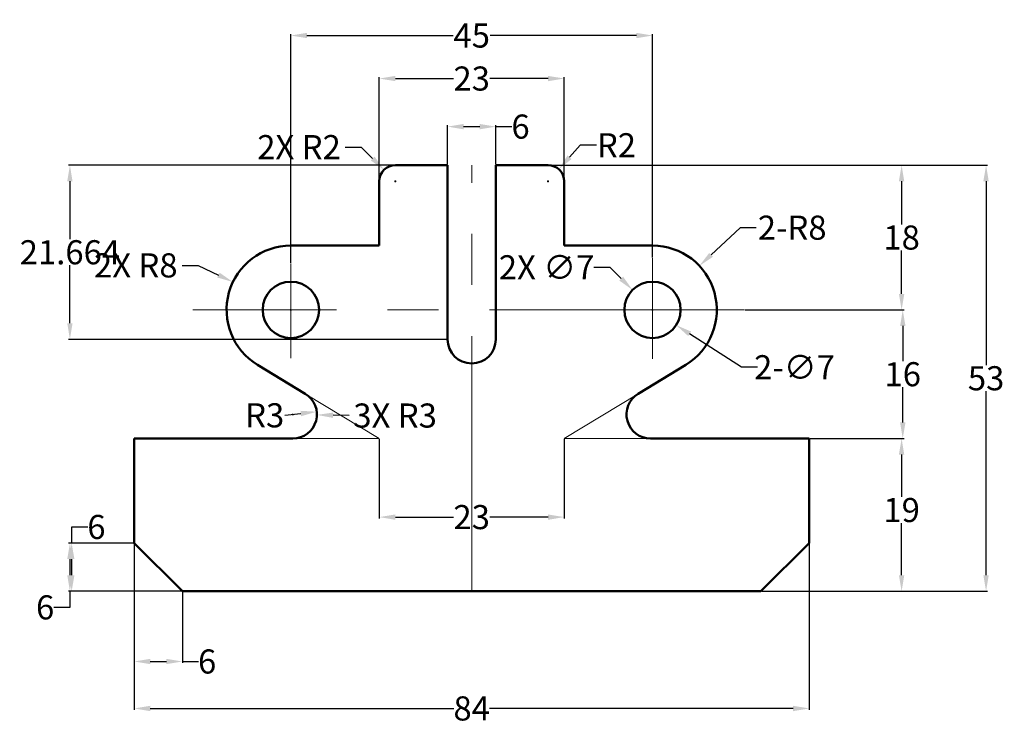
# Model space of a CAD drawing. Units: inches. Extents: x 46 to 168, y 15 to 102.
import ezdxf

# ---------------------------------------------------------------- set-up
doc = ezdxf.new("R2010")
doc.units = ezdxf.units.IN
doc.header["$MEASUREMENT"] = 0
doc.linetypes.add('ACAD_ISO04W100', pattern=[30, 24, -3, 0, -3])
doc.linetypes.add('CENTER', pattern=[50.8, 31.75, -6.35, 6.35, -6.35])
for name, color, linetype, lineweight in [('M-CNTR', 4, 'CENTER', 18), ('M-CONS', 4, 'ACAD_ISO04W100', 18), ('M-DIMS', 2, 'Continuous', 25), ('M-OUTL', 7, 'Continuous', 50)]:
    doc.layers.add(name, color=color, linetype=linetype, lineweight=lineweight)
doc.styles.get("Standard").update_dxf_attribs({"font": 'arial.ttf'})
doc.dimstyles.get("Standard").update_dxf_attribs({"dimtxt": 3, "dimasz": 2, "dimexe": 0.18, "dimexo": 0.0625, "dimgap": 0.09, "dimtad": 0, "dimtih": 1, "dimtoh": 1, "dimdec": 0, "dimzin": 0, "dimdsep": 46, "dimtxsty": 'Standard', "dimcen": 0.09, "dimclrd": 1, "dimclre": 1, "dimadec": 0, "dimazin": 0, "dimtfac": 1, "dimtdec": 0, "dimtofl": 0, "dimtmove": 0, "dimatfit": 3, "dimfxl": 1, "dimtolj": 1, "dimtzin": 0, "dimarcsym": 0})

# ---------------------------------------------------------------- blocks, each defined once
blk = doc.blocks.new('*D1')
at = {"layer": 'Defpoints', "color": 0, "transparency": 16777216}
for p in [(144.16, 50.26), (138.16, 31.26), (155.66, 31.26)]:
    blk.add_point(p, dxfattribs=at)
at = {"layer": 'M-DIMS', "color": 0, "lineweight": -2, "transparency": 16777216}
for p, q in [((144.22, 50.26), (155.84, 50.26)), ((155.66, 48.26), (155.66, 42.99)), ((155.66, 33.26), (155.66, 39.75)), ((138.22, 31.26), (155.84, 31.26))]:
    blk.add_line(p, q, dxfattribs=at)
at = {"layer": 'M-DIMS', "color": 0, "transparency": 16777216}
for points in [[(155.32, 48.26), (155.99, 48.26), (155.66, 50.26)], [(155.32, 33.26), (155.99, 33.26), (155.66, 31.26)]]:
    blk.add_solid(points, dxfattribs=at)
at = {"layer": 'M-DIMS', "color": 0, "transparency": 16777216, "insert": (155.66, 41.37), "char_height": 3, "attachment_point": 5}
blk.add_mtext('\\A1;19', dxfattribs=at)
blk = doc.blocks.new('*D2')
at = {"layer": 'Defpoints', "color": 0, "transparency": 16777216}
for p in [(60.16, 37.26), (66.16, 31.26), (66.16, 22.53)]:
    blk.add_point(p, dxfattribs=at)
at = {"layer": 'M-DIMS', "color": 0, "lineweight": -2, "transparency": 16777216}
for p, q in [((60.16, 37.2), (60.16, 22.35)), ((66.16, 31.2), (66.16, 22.35)), ((62.16, 22.53), (64.16, 22.53)), ((66.16, 22.53), (68.16, 22.53))]:
    blk.add_line(p, q, dxfattribs=at)
at = {"layer": 'M-DIMS', "color": 0, "transparency": 16777216}
for points in [[(62.16, 22.86), (62.16, 22.2), (60.16, 22.53)], [(64.16, 22.86), (64.16, 22.2), (66.16, 22.53)]]:
    blk.add_solid(points, dxfattribs=at)
at = {"layer": 'M-DIMS', "color": 0, "transparency": 16777216, "insert": (69.24, 22.53), "char_height": 3, "attachment_point": 5}
blk.add_mtext('\\A1;6', dxfattribs=at)
blk = doc.blocks.new('*D3')
at = {"layer": 'Defpoints', "color": 0, "transparency": 16777216}
for p in [(52.38, 37.26), (60.16, 37.26), (66.16, 31.26)]:
    blk.add_point(p, dxfattribs=at)
at = {"layer": 'M-DIMS', "color": 0, "lineweight": -2, "transparency": 16777216}
for p, q in [((52.38, 37.26), (52.38, 39.26)), ((52.38, 39.26), (54.38, 39.26)), ((60.1, 37.26), (52.2, 37.26)), ((52.38, 33.26), (52.38, 35.26)), ((66.1, 31.26), (52.2, 31.26))]:
    blk.add_line(p, q, dxfattribs=at)
at = {"layer": 'M-DIMS', "color": 0, "transparency": 16777216}
for points in [[(52.05, 35.26), (52.72, 35.26), (52.38, 37.26)], [(52.05, 33.26), (52.72, 33.26), (52.38, 31.26)]]:
    blk.add_solid(points, dxfattribs=at)
at = {"layer": 'M-DIMS', "color": 0, "transparency": 16777216, "insert": (55.46, 39.26), "char_height": 3, "attachment_point": 5}
blk.add_mtext('\\A1;6', dxfattribs=at)
blk = doc.blocks.new('*D4')
at = {"layer": 'Defpoints', "color": 0, "transparency": 16777216}
for p in [(136.12, 66.26), (144.16, 50.26), (155.8, 50.26)]:
    blk.add_point(p, dxfattribs=at)
at = {"layer": 'M-DIMS', "color": 0, "lineweight": -2, "transparency": 16777216}
for p, q in [((136.18, 66.26), (155.98, 66.26)), ((155.8, 64.26), (155.8, 59.89)), ((155.8, 52.26), (155.8, 56.64)), ((144.22, 50.26), (155.98, 50.26))]:
    blk.add_line(p, q, dxfattribs=at)
at = {"layer": 'M-DIMS', "color": 0, "transparency": 16777216}
for points in [[(155.47, 64.26), (156.14, 64.26), (155.8, 66.26)], [(155.47, 52.26), (156.14, 52.26), (155.8, 50.26)]]:
    blk.add_solid(points, dxfattribs=at)
at = {"layer": 'M-DIMS', "color": 0, "transparency": 16777216, "insert": (155.8, 58.26), "char_height": 3, "attachment_point": 5}
blk.add_mtext('\\A1;16', dxfattribs=at)
blk = doc.blocks.new('*D5')
at = {"layer": 'Defpoints', "color": 0, "transparency": 16777216}
for p in [(111.66, 84.26), (136.12, 66.26), (155.66, 66.26)]:
    blk.add_point(p, dxfattribs=at)
at = {"layer": 'M-DIMS', "color": 0, "lineweight": -2, "transparency": 16777216}
for p, q in [((111.72, 84.26), (155.84, 84.26)), ((155.66, 82.26), (155.66, 76.89)), ((155.66, 68.26), (155.66, 73.64)), ((136.18, 66.26), (155.84, 66.26))]:
    blk.add_line(p, q, dxfattribs=at)
at = {"layer": 'M-DIMS', "color": 0, "transparency": 16777216}
for points in [[(155.32, 82.26), (155.99, 82.26), (155.66, 84.26)], [(155.32, 68.26), (155.99, 68.26), (155.66, 66.26)]]:
    blk.add_solid(points, dxfattribs=at)
at = {"layer": 'M-DIMS', "color": 0, "transparency": 16777216, "insert": (155.66, 75.26), "char_height": 3, "attachment_point": 5}
blk.add_mtext('\\A1;18', dxfattribs=at)
blk = doc.blocks.new('*D6')
at = {"layer": 'Defpoints', "color": 0, "transparency": 16777216}
for p in [(105.16, 89.06), (99.16, 84.26), (105.16, 84.26)]:
    blk.add_point(p, dxfattribs=at)
at = {"layer": 'M-DIMS', "color": 0, "lineweight": -2, "transparency": 16777216}
for p, q in [((99.16, 84.33), (99.16, 89.24)), ((101.16, 89.06), (103.16, 89.06)), ((105.16, 84.33), (105.16, 89.24)), ((105.16, 89.06), (107.16, 89.06))]:
    blk.add_line(p, q, dxfattribs=at)
at = {"layer": 'M-DIMS', "color": 0, "transparency": 16777216}
for points in [[(101.16, 89.39), (101.16, 88.72), (99.16, 89.06)], [(103.16, 89.39), (103.16, 88.72), (105.16, 89.06)]]:
    blk.add_solid(points, dxfattribs=at)
at = {"layer": 'M-DIMS', "color": 0, "transparency": 16777216, "insert": (108.24, 89.06), "char_height": 3, "attachment_point": 5}
blk.add_mtext('\\A1;6', dxfattribs=at)
blk = doc.blocks.new('*D7')
at = {"layer": 'Defpoints', "color": 0, "transparency": 16777216}
for p in [(111.66, 84.26), (138.16, 31.26), (166.17, 31.26)]:
    blk.add_point(p, dxfattribs=at)
at = {"layer": 'M-DIMS', "color": 0, "lineweight": -2, "transparency": 16777216}
for p, q in [((111.72, 84.26), (166.35, 84.26)), ((166.17, 82.26), (166.17, 59.39)), ((166.17, 33.26), (166.17, 56.14)), ((138.22, 31.26), (166.35, 31.26))]:
    blk.add_line(p, q, dxfattribs=at)
at = {"layer": 'M-DIMS', "color": 0, "transparency": 16777216}
for points in [[(165.83, 82.26), (166.5, 82.26), (166.17, 84.26)], [(165.83, 33.26), (166.5, 33.26), (166.17, 31.26)]]:
    blk.add_solid(points, dxfattribs=at)
at = {"layer": 'M-DIMS', "color": 0, "transparency": 16777216, "insert": (166.17, 57.76), "char_height": 3, "attachment_point": 5}
blk.add_mtext('\\A1;53', dxfattribs=at)
blk = doc.blocks.new('*D8')
at = {"layer": 'Defpoints', "color": 0, "transparency": 16777216}
for p in [(130.49, 71.74), (124.66, 66.26)]:
    blk.add_point(p, dxfattribs=at)
at = {"layer": 'M-DIMS', "color": 0, "lineweight": -2, "transparency": 16777216}
for p, q in [((135.56, 76.49), (131.95, 73.1)), ((137.56, 76.49), (135.56, 76.49)), ((124.57, 66.26), (124.75, 66.26)), ((124.66, 66.17), (124.66, 66.35))]:
    blk.add_line(p, q, dxfattribs=at)
at = {"layer": 'M-DIMS', "color": 0, "transparency": 16777216}
blk.add_solid([(131.72, 73.35), (132.18, 72.86), (130.49, 71.74)], dxfattribs=at)
at = {"layer": 'M-DIMS', "color": 0, "transparency": 16777216, "insert": (142.04, 76.49), "char_height": 3, "attachment_point": 5}
blk.add_mtext('\\A1;2-R8', dxfattribs=at)
blk = doc.blocks.new('*D9')
at = {"layer": 'Defpoints', "color": 0, "transparency": 16777216}
for p in [(121.72, 68.16), (127.6, 64.37)]:
    blk.add_point(p, dxfattribs=at)
at = {"layer": 'M-DIMS', "color": 0, "lineweight": -2, "transparency": 16777216}
for p, q in [((124.57, 66.26), (124.75, 66.26)), ((124.66, 66.17), (124.66, 66.35)), ((135.73, 59.13), (129.28, 63.29)), ((137.73, 59.13), (135.73, 59.13))]:
    blk.add_line(p, q, dxfattribs=at)
at = {"layer": 'M-DIMS', "color": 0, "transparency": 16777216}
blk.add_solid([(129.46, 63.57), (129.1, 63.01), (127.6, 64.37)], dxfattribs=at)
at = {"layer": 'M-DIMS', "color": 0, "transparency": 16777216, "insert": (142.33, 59.13), "char_height": 3, "attachment_point": 5}
blk.add_mtext('\\A1;2-∅7', dxfattribs=at)
blk = doc.blocks.new('*D10')
at = {"layer": 'Defpoints', "color": 0, "transparency": 16777216}
for p in [(60.16, 37.26), (144.16, 37.26), (144.16, 16.69)]:
    blk.add_point(p, dxfattribs=at)
at = {"layer": 'M-DIMS', "color": 0, "lineweight": -2, "transparency": 16777216}
for p, q in [((60.16, 37.2), (60.16, 16.51)), ((144.16, 37.2), (144.16, 16.51)), ((62.16, 16.69), (99.92, 16.69)), ((142.16, 16.69), (104.39, 16.69))]:
    blk.add_line(p, q, dxfattribs=at)
at = {"layer": 'M-DIMS', "color": 0, "transparency": 16777216}
for points in [[(62.16, 17.02), (62.16, 16.35), (60.16, 16.69)], [(142.16, 17.02), (142.16, 16.35), (144.16, 16.69)]]:
    blk.add_solid(points, dxfattribs=at)
at = {"layer": 'M-DIMS', "color": 0, "transparency": 16777216, "insert": (102.16, 16.69), "char_height": 3, "attachment_point": 5}
blk.add_mtext('\\A1;84', dxfattribs=at)
blk = doc.blocks.new('*D11')
at = {"layer": 'Defpoints', "color": 0, "transparency": 16777216}
for p in [(124.66, 100.39), (124.66, 72.7), (79.66, 72.05)]:
    blk.add_point(p, dxfattribs=at)
at = {"layer": 'M-DIMS', "color": 0, "lineweight": -2, "transparency": 16777216}
for p, q in [((79.66, 72.12), (79.66, 100.57)), ((124.66, 72.76), (124.66, 100.57)), ((81.66, 100.39), (99.85, 100.39)), ((122.66, 100.39), (104.47, 100.39))]:
    blk.add_line(p, q, dxfattribs=at)
at = {"layer": 'M-DIMS', "color": 0, "transparency": 16777216}
for points in [[(81.66, 100.72), (81.66, 100.06), (79.66, 100.39)], [(122.66, 100.72), (122.66, 100.06), (124.66, 100.39)]]:
    blk.add_solid(points, dxfattribs=at)
at = {"layer": 'M-DIMS', "color": 0, "transparency": 16777216, "insert": (102.16, 100.39), "char_height": 3, "attachment_point": 5}
blk.add_mtext('\\A1;45', dxfattribs=at)
blk = doc.blocks.new('*D12')
at = {"layer": 'Defpoints', "color": 0, "transparency": 16777216}
for p in [(113.66, 95.04), (90.66, 82.26), (113.66, 82.26)]:
    blk.add_point(p, dxfattribs=at)
at = {"layer": 'M-DIMS', "color": 0, "lineweight": -2, "transparency": 16777216}
for p, q in [((90.66, 82.33), (90.66, 95.22)), ((92.66, 95.04), (99.89, 95.04)), ((111.66, 95.04), (104.42, 95.04)), ((113.66, 82.33), (113.66, 95.22))]:
    blk.add_line(p, q, dxfattribs=at)
at = {"layer": 'M-DIMS', "color": 0, "transparency": 16777216}
for points in [[(92.66, 95.37), (92.66, 94.71), (90.66, 95.04)], [(111.66, 95.37), (111.66, 94.71), (113.66, 95.04)]]:
    blk.add_solid(points, dxfattribs=at)
at = {"layer": 'M-DIMS', "color": 0, "transparency": 16777216, "insert": (102.16, 95.04), "char_height": 3, "attachment_point": 5}
blk.add_mtext('\\A1;23', dxfattribs=at)
blk = doc.blocks.new('*D13')
at = {"layer": 'Defpoints', "color": 0, "transparency": 16777216}
for p in [(112.99, 83.75), (111.66, 82.26)]:
    blk.add_point(p, dxfattribs=at)
at = {"layer": 'M-DIMS', "color": 0, "lineweight": -2, "transparency": 16777216}
for p, q in [((115.67, 86.74), (114.33, 85.24)), ((117.67, 86.74), (115.67, 86.74)), ((111.57, 82.26), (111.75, 82.26)), ((111.66, 82.17), (111.66, 82.35))]:
    blk.add_line(p, q, dxfattribs=at)
at = {"layer": 'M-DIMS', "color": 0, "transparency": 16777216}
blk.add_solid([(114.08, 85.47), (114.58, 85.02), (112.99, 83.75)], dxfattribs=at)
at = {"layer": 'M-DIMS', "color": 0, "transparency": 16777216, "insert": (120.17, 86.74), "char_height": 3, "attachment_point": 5}
blk.add_mtext('\\A1;R2', dxfattribs=at)
blk = doc.blocks.new('*D14')
at = {"layer": 'Defpoints', "color": 0, "transparency": 16777216}
for p in [(90.66, 50.26), (113.66, 50.26), (113.66, 40.49)]:
    blk.add_point(p, dxfattribs=at)
at = {"layer": 'M-DIMS', "color": 0, "lineweight": -2, "transparency": 16777216}
for p, q in [((90.66, 50.2), (90.66, 40.31)), ((113.66, 50.2), (113.66, 40.31)), ((92.66, 40.49), (99.89, 40.49)), ((111.66, 40.49), (104.42, 40.49))]:
    blk.add_line(p, q, dxfattribs=at)
at = {"layer": 'M-DIMS', "color": 0, "transparency": 16777216}
for points in [[(92.66, 40.82), (92.66, 40.15), (90.66, 40.49)], [(111.66, 40.82), (111.66, 40.15), (113.66, 40.49)]]:
    blk.add_solid(points, dxfattribs=at)
at = {"layer": 'M-DIMS', "color": 0, "transparency": 16777216, "insert": (102.16, 40.49), "char_height": 3, "attachment_point": 5}
blk.add_mtext('\\A1;23', dxfattribs=at)
blk = doc.blocks.new('*D15')
at = {"layer": 'Defpoints', "color": 0, "transparency": 16777216}
for p in [(79.9, 53.26), (82.88, 53.6)]:
    blk.add_point(p, dxfattribs=at)
at = {"layer": 'M-DIMS', "color": 0, "lineweight": -2, "transparency": 16777216}
blk.add_line((78.91, 53.15), (80.89, 53.37), dxfattribs=at)
at = {"layer": 'M-DIMS', "color": 0, "transparency": 16777216}
blk.add_solid([(80.86, 53.71), (80.93, 53.04), (82.88, 53.6)], dxfattribs=at)
at = {"layer": 'M-DIMS', "color": 0, "transparency": 16777216, "insert": (76.4, 53.15), "char_height": 3, "attachment_point": 5}
blk.add_mtext('\\A1;R3', dxfattribs=at)
blk = doc.blocks.new('LINK-THRU-HOLE-D7')
blk.add_circle((3.5, 3.5), 3.5)
blk = doc.blocks.new('*D17')
at = {"layer": 'Defpoints', "color": 0, "transparency": 16777216}
for p in [(99.16, 84.26), (52.16, 62.6), (99.16, 62.6)]:
    blk.add_point(p, dxfattribs=at)
at = {"layer": 'M-DIMS', "color": 1, "lineweight": -2, "transparency": 16777216}
for p, q in [((99.1, 84.26), (51.98, 84.26)), ((52.16, 82.26), (52.16, 75.05)), ((52.16, 64.6), (52.16, 71.81)), ((99.1, 62.6), (51.98, 62.6))]:
    blk.add_line(p, q, dxfattribs=at)
at = {"layer": 'M-DIMS', "color": 1, "transparency": 16777216}
for points in [[(51.83, 82.26), (52.49, 82.26), (52.16, 84.26)], [(51.83, 64.6), (52.49, 64.6), (52.16, 62.6)]]:
    blk.add_solid(points, dxfattribs=at)
at = {"layer": 'M-DIMS', "color": 0, "transparency": 16777216, "insert": (52.16, 73.43), "char_height": 3, "attachment_point": 5}
blk.add_mtext('\\A1;21.664', dxfattribs=at)
blk = doc.blocks.new('*D18')
at = {"layer": 'Defpoints', "color": 0, "transparency": 16777216}
for p in [(60.16, 37.26), (52.16, 31.26), (66.16, 31.26)]:
    blk.add_point(p, dxfattribs=at)
at = {"layer": 'M-DIMS', "color": 1, "lineweight": -2, "transparency": 16777216}
for p, q in [((60.1, 37.26), (51.98, 37.26)), ((52.16, 35.26), (52.16, 33.26)), ((66.1, 31.26), (51.98, 31.26)), ((52.16, 31.26), (52.16, 29.26)), ((52.16, 29.26), (50.16, 29.26))]:
    blk.add_line(p, q, dxfattribs=at)
at = {"layer": 'M-DIMS', "color": 1, "transparency": 16777216}
for points in [[(51.83, 35.26), (52.49, 35.26), (52.16, 37.26)], [(51.83, 33.26), (52.49, 33.26), (52.16, 31.26)]]:
    blk.add_solid(points, dxfattribs=at)
at = {"layer": 'M-DIMS', "color": 0, "transparency": 16777216, "insert": (49.08, 29.26), "char_height": 3, "attachment_point": 5}
blk.add_mtext('\\A1;6', dxfattribs=at)
blk = doc.blocks.new('*D19')
at = {"layer": 'Defpoints', "color": 0, "transparency": 16777216}
for p in [(72.45, 69.73), (79.66, 66.26)]:
    blk.add_point(p, dxfattribs=at)
at = {"layer": 'M-DIMS', "color": 1, "lineweight": -2, "transparency": 16777216}
for p, q in [((66.12, 71.8), (68.12, 71.8)), ((68.12, 71.8), (70.64, 70.59)), ((79.57, 66.26), (79.75, 66.26)), ((79.66, 66.17), (79.66, 66.35))]:
    blk.add_line(p, q, dxfattribs=at)
at = {"layer": 'M-DIMS', "color": 1, "transparency": 16777216}
blk.add_solid([(70.79, 70.89), (70.5, 70.29), (72.45, 69.73)], dxfattribs=at)
at = {"layer": 'M-DIMS', "color": 0, "transparency": 16777216, "insert": (60.36, 71.8), "char_height": 3, "attachment_point": 5}
blk.add_mtext('\\A1;2X R8', dxfattribs=at)
blk = doc.blocks.new('*D20')
at = {"layer": 'Defpoints', "color": 0, "transparency": 16777216}
for p in [(122.18, 68.74), (127.14, 63.79)]:
    blk.add_point(p, dxfattribs=at)
at = {"layer": 'M-DIMS', "color": 1, "lineweight": -2, "transparency": 16777216}
for p, q in [((117.35, 71.56), (119.35, 71.56)), ((119.35, 71.56), (120.77, 70.15)), ((124.57, 66.26), (124.75, 66.26)), ((124.66, 66.17), (124.66, 66.35))]:
    blk.add_line(p, q, dxfattribs=at)
at = {"layer": 'M-DIMS', "color": 1, "transparency": 16777216}
blk.add_solid([(121, 70.39), (120.53, 69.91), (122.18, 68.74)], dxfattribs=at)
at = {"layer": 'M-DIMS', "color": 0, "transparency": 16777216, "insert": (111.48, 71.56), "char_height": 3, "attachment_point": 5}
blk.add_mtext('\\A1;2X ∅7', dxfattribs=at)
blk = doc.blocks.new('*D21')
at = {"layer": 'Defpoints', "color": 0, "transparency": 16777216}
for p in [(79.9, 53.26), (82.9, 53.2)]:
    blk.add_point(p, dxfattribs=at)
at = {"layer": 'M-DIMS', "color": 1, "lineweight": -2, "transparency": 16777216}
for p, q in [((79.81, 53.26), (79.99, 53.26)), ((79.9, 53.17), (79.9, 53.35)), ((86.9, 53.12), (84.9, 53.16))]:
    blk.add_line(p, q, dxfattribs=at)
at = {"layer": 'M-DIMS', "color": 1, "transparency": 16777216}
blk.add_solid([(84.91, 53.49), (84.89, 52.83), (82.9, 53.2)], dxfattribs=at)
at = {"layer": 'M-DIMS', "color": 0, "transparency": 16777216, "insert": (92.63, 53.12), "char_height": 3, "attachment_point": 5}
blk.add_mtext('\\A1;3X R3', dxfattribs=at)
blk = doc.blocks.new('*D22')
at = {"layer": 'Defpoints', "color": 0, "transparency": 16777216}
for p in [(91.24, 83.68), (92.66, 82.26)]:
    blk.add_point(p, dxfattribs=at)
at = {"layer": 'M-DIMS', "color": 1, "lineweight": -2, "transparency": 16777216}
for p, q in [((86.42, 86.51), (88.42, 86.51)), ((88.42, 86.51), (89.83, 85.09)), ((92.57, 82.26), (92.75, 82.26)), ((92.66, 82.17), (92.66, 82.35))]:
    blk.add_line(p, q, dxfattribs=at)
at = {"layer": 'M-DIMS', "color": 1, "transparency": 16777216}
blk.add_solid([(90.07, 85.33), (89.59, 84.86), (91.24, 83.68)], dxfattribs=at)
at = {"layer": 'M-DIMS', "color": 0, "transparency": 16777216, "insert": (80.67, 86.51), "char_height": 3, "attachment_point": 5}
blk.add_mtext('\\A1;2X R2', dxfattribs=at)

msp = doc.modelspace()

# ---------------------------------------------------------------- linework, layer by layer
at = {"layer": 'M-CNTR'}
for p, q in [((102.1592, 31.2639), (102.1592, 84.2639)), ((124.6592, 60.1911), (124.6592, 72.6961)), ((79.6592, 60.2495), (79.6592, 72.0533)), ((136.1203, 66.2639), (67.441, 66.2639))]:
    msp.add_line(p, q, dxfattribs=at)
at = {"layer": 'M-CONS'}
for p, q in [((81.452, 55.8311), (90.6592, 50.2639)), ((122.8663, 55.8311), (113.6592, 50.2639)), ((79.8997, 50.2639), (90.6592, 50.2639)), ((124.4186, 50.2639), (113.6592, 50.2639))]:
    msp.add_line(p, q, dxfattribs=at)
at = {"layer": 'M-OUTL'}
for p, q in [((99.1592, 66.2639), (99.1592, 84.2639)), ((105.1592, 66.2639), (105.1592, 84.2639)), ((105.1592, 84.2639), (111.6592, 84.2639)), ((113.6592, 82.2639), (113.6592, 74.2639)), ((79.6592, 74.2639), (90.6592, 74.2639)), ((124.6592, 74.2639), (113.6592, 74.2639)), ((99.1592, 66.2639), (99.1592, 62.6004)), ((105.1592, 66.2639), (105.1592, 62.6004)), ((81.452, 55.8311), (75.5198, 59.4181)), ((122.8663, 55.8311), (128.7985, 59.4181)), ((60.1592, 37.2639), (60.1592, 50.2639)), ((60.1592, 50.2639), (79.8997, 50.2639)), ((144.1592, 50.2639), (124.4186, 50.2639)), ((144.1592, 37.2639), (144.1592, 50.2639)), ((66.1592, 31.2639), (60.1592, 37.2639)), ((138.1592, 31.2639), (144.1592, 37.2639)), ((66.1592, 31.2639), (138.1592, 31.2639))]:
    msp.add_line(p, q, dxfattribs=at)
msp.add_lwpolyline([(99.1592, 84.2639), (94.6592, 84.2639), (92.6592, 84.2639, 0.41421356), (90.6592, 82.2639), (90.6592, 80.2639), (90.6592, 74.2639)], format="xyb", dxfattribs=at)
for centre, radius, start, end in [((111.6592, 82.2639), 2, 0, 90), ((79.6592, 66.2639), 8, 90, 238.840375), ((124.6592, 66.2639), 8, 301.159625, 90), ((102.1592, 62.6004), 3, 180, 0), ((79.8997, 53.2639), 3, 270, 58.840375), ((124.4186, 53.2639), 3, 121.159625, 270)]:
    msp.add_arc(centre, radius, start, end, dxfattribs=at)

# ---------------------------------------------------------------- block references
for p in [(76.159, 62.764), (121.159, 62.764)]:
    msp.add_blockref('LINK-THRU-HOLE-D7', p, dxfattribs=at)

# ---------------------------------------------------------------- dimensions: what is measured, and where the dimension line sits
at = {"layer": 'M-DIMS'}
for base, p1, p2, picture, middle in [((124.6592, 100.3893), (79.6592, 72.0533), (124.6592, 72.6961), '*D11', (102.1592, 100.3893)), ((113.6592, 95.0417), (90.6592, 82.2639), (113.6592, 82.2639), '*D12', (102.1592, 95.0417)), ((113.6592, 40.4852), (90.6592, 50.2639), (113.6592, 50.2639), '*D14', (102.1592, 40.4852)), ((66.1592, 22.5292), (60.1592, 37.2639), (66.1592, 31.2639), '*D2', (69.2396, 22.5292)), ((144.1592, 16.6859), (60.1592, 37.2639), (144.1592, 37.2639), '*D10', (102.1592, 16.6859))]:
    dim = msp.add_linear_dim(base=base, p1=p1, p2=p2, dimstyle='Standard', override={"dimclrd": 0, "dimclre": 0, "dimclrt": 0}, dxfattribs=at)
    dim.commit()
    dim.dimension.update_dxf_attribs({"geometry": picture, "text_midpoint": middle})
for center, mpoint, text, picture, middle in [((92.6592, 82.2639), (91.2449, 83.6781), '2X <>', '*D22', (80.6743, 86.5064)), ((79.8997, 53.2639), (82.8991, 53.2021), '3X <>', '*D21', (92.6291, 53.1196))]:
    dim = msp.add_radius_dim(center=center, mpoint=mpoint, text=text, dimstyle='Standard', override={"dimdec": 0, "dimlfac": 1, "dimrnd": 0, "dimzin": 0, "dimdsep": 46, "dimlunit": 2}, dxfattribs=at)
    dim.commit()
    dim.dimension.update_dxf_attribs({"geometry": picture, "text_midpoint": middle})
for base, p1, p2, angle, override, picture, middle in [((105.1592, 89.0577), (99.1592, 84.2639), (105.1592, 84.2639), 180, {"dimclrd": 0, "dimclre": 0, "dimclrt": 0}, '*D6', (108.2396, 89.0577)), ((52.15915, 62.6004), (99.15915, 84.26393), (99.15915, 62.60039), 90, {"dimdec": 3, "dimlfac": 1, "dimrnd": 0, "dimzin": 0, "dimdsep": 46, "dimlunit": 2}, '*D17', (52.15915, 73.43216)), ((52.1592, 31.2639), (60.1592, 37.2639), (66.1592, 31.2639), 90, {"dimdec": 0, "dimlfac": 1, "dimrnd": 0, "dimzin": 0, "dimdsep": 46, "dimlunit": 2}, '*D18', (49.0787, 29.2639))]:
    dim = msp.add_linear_dim(base=base, p1=p1, p2=p2, angle=angle, dimstyle='Standard', override=override, dxfattribs=at)
    dim.commit()
    dim.dimension.update_dxf_attribs({"geometry": picture, "text_midpoint": middle})
for center, mpoint, picture, middle in [((111.6592, 82.2639), (112.994, 83.7533), '*D13', (120.1665, 86.7425)), ((79.8997, 53.2639), (82.8812, 53.5965), '*D15', (78.9059, 53.1531))]:
    dim = msp.add_radius_dim(center=center, mpoint=mpoint, dimstyle='Standard', override={"dimclrd": 0, "dimclre": 0, "dimclrt": 0}, dxfattribs=at)
    dim.commit()
    dim.dimension.update_dxf_attribs({"geometry": picture, "text_midpoint": middle, "dimtype": 164})
for base, p1, p2, picture, middle in [((155.6557, 66.2639), (111.6592, 84.2639), (136.1203, 66.2639), '*D5', (155.6557, 75.2639)), ((166.1663, 31.2639), (111.6592, 84.2639), (138.1592, 31.2639), '*D7', (166.1663, 57.7639)), ((155.8017, 50.2639), (136.1203, 66.2639), (144.1592, 50.2639), '*D4', (155.8017, 58.2639)), ((155.6557, 31.2639), (144.1592, 50.2639), (138.1592, 31.2639), '*D1', (155.6557, 41.3732)), ((52.3829, 37.2639), (66.1592, 31.2639), (60.1592, 37.2639), '*D3', (55.4633, 39.2639))]:
    dim = msp.add_linear_dim(base=base, p1=p1, p2=p2, angle=90, dimstyle='Standard', override={"dimclrd": 0, "dimclre": 0, "dimclrt": 0}, dxfattribs=at)
    dim.commit()
    dim.dimension.update_dxf_attribs({"geometry": picture, "text_midpoint": middle, "dimtype": 160})
for center, mpoint, text, override, picture, middle in [((124.6592, 66.2639), (130.4942, 71.7368), '2-<>', {"dimclrd": 0, "dimclre": 0, "dimclrt": 0}, '*D8', (142.0431, 76.4924)), ((79.6592, 66.2639), (72.4468, 69.7255), '2X <>', {"dimdec": 0, "dimlfac": 1, "dimrnd": 0, "dimzin": 0, "dimdsep": 46, "dimlunit": 2}, '*D19', (60.3589, 71.8025))]:
    dim = msp.add_radius_dim(center=center, mpoint=mpoint, text=text, dimstyle='Standard', override=override, dxfattribs=at)
    dim.commit()
    dim.dimension.update_dxf_attribs({"geometry": picture, "text_midpoint": middle, "dimtype": 164})
for p1, p2, text, override, picture, middle in [((127.1356, 63.7906), (122.1827, 68.7373), '2X <>', {"dimdec": 0, "dimlfac": 1, "dimrnd": 0, "dimzin": 0, "dimdsep": 46, "dimlunit": 2}, '*D20', (111.4784, 71.5639)), ((121.7165, 68.1589), (127.6018, 64.3689), '2-<>', {"dimclrd": 0, "dimclre": 0, "dimclrt": 0}, '*D9', (142.3258, 59.132))]:
    dim = msp.add_diameter_dim_2p(p1=p1, p2=p2, text=text, dimstyle='Standard', override=override, dxfattribs=at)
    dim.commit()
    dim.dimension.update_dxf_attribs({"geometry": picture, "text_midpoint": middle, "dimtype": 163})

doc.saveas('drawing.dxf')
